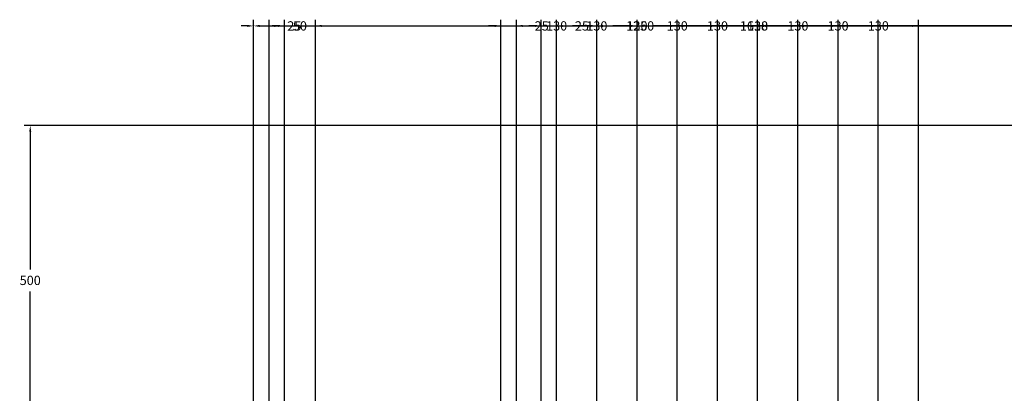
# Model space of a CAD drawing. Units: millimetres. Extents: x 937 to 4561, y 2711 to 5748.
# Tile 4 of 8: x 951 to 2543, y 5145 to 5748. Entities that reach past the tile are written whole.
import ezdxf

# ---------------------------------------------------------------- set-up
doc = ezdxf.new("R2010")
doc.units = ezdxf.units.MM
doc.header["$MEASUREMENT"] = 0
doc.layers.add('A-ANNO-DIMS', color=2, linetype='Continuous', lineweight=18)
doc.styles.get("Standard").update_dxf_attribs({"font": 'arial.ttf'})
doc.dimstyles.get("Standard").update_dxf_attribs({"dimtxt": 15, "dimasz": 10, "dimexe": 10, "dimexo": 10, "dimgap": 10, "dimtad": 0, "dimtih": 1, "dimtoh": 1, "dimdec": 0, "dimzin": 0, "dimdsep": 46, "dimtxsty": 'Standard', "dimcen": 5, "dimadec": 0, "dimazin": 0, "dimtfac": 1, "dimtdec": 0, "dimtofl": 0, "dimtmove": 0, "dimatfit": 3, "dimfxl": 1, "dimtolj": 1, "dimtzin": 0, "dimarcsym": 0})

# ---------------------------------------------------------------- blocks, each defined once
blk = doc.blocks.new('*D15')
at = {"layer": 'A-ANNO-DIMS', "color": 0, "lineweight": -2, "transparency": 16777216}
for p, q in [((1329.5, 4086.9), (1329.5, 5747.9)), ((4179.5, 5586.9), (4179.5, 5747.9)), ((1339.5, 5737.9), (2722, 5737.9)), ((4169.5, 5737.9), (2787, 5737.9))]:
    blk.add_line(p, q, dxfattribs=at)
at = {"layer": 'A-ANNO-DIMS', "color": 0, "transparency": 16777216}
for points in [[(1339.5, 5739.6), (1339.5, 5736.2), (1329.5, 5737.9)], [(4169.5, 5739.6), (4169.5, 5736.2), (4179.5, 5737.9)]]:
    blk.add_solid(points, dxfattribs=at)
at = {"layer": 'Defpoints', "color": 0, "transparency": 16777216}
for p in [(4179.5, 5737.9), (4179.5, 5576.9), (1329.5, 4076.9)]:
    blk.add_point(p, dxfattribs=at)
at = {"layer": 'A-ANNO-DIMS', "color": 0, "transparency": 16777216, "insert": (2754.5, 5737.9), "char_height": 15, "attachment_point": 5}
blk.add_mtext('\\A1;2850', dxfattribs=at)
blk = doc.blocks.new('*D16')
at = {"layer": 'A-ANNO-DIMS', "color": 0, "lineweight": -2, "transparency": 16777216}
for p, q in [((1329.5, 4859.2), (1329.5, 5747.9)), ((2947.4, 5137.7), (2947.4, 5747.9)), ((1339.5, 5737.9), (2106.8, 5737.9)), ((2937.4, 5737.9), (2170.2, 5737.9))]:
    blk.add_line(p, q, dxfattribs=at)
at = {"layer": 'A-ANNO-DIMS', "color": 0, "transparency": 16777216}
for points in [[(1339.5, 5739.6), (1339.5, 5736.2), (1329.5, 5737.9)], [(2937.4, 5739.6), (2937.4, 5736.2), (2947.4, 5737.9)]]:
    blk.add_solid(points, dxfattribs=at)
at = {"layer": 'Defpoints', "color": 0, "transparency": 16777216}
for p in [(2947.4, 5737.9), (2947.4, 5127.7), (1329.5, 4849.2)]:
    blk.add_point(p, dxfattribs=at)
at = {"layer": 'A-ANNO-DIMS', "color": 0, "transparency": 16777216, "insert": (2138.5, 5737.9), "char_height": 15, "attachment_point": 5}
blk.add_mtext('\\A1;1618', dxfattribs=at)
blk = doc.blocks.new('*D20')
at = {"layer": 'A-ANNO-DIMS', "color": 0, "lineweight": -2, "transparency": 16777216}
for p, q in [((1379.5, 5086.9), (1379.5, 5747.9)), ((1429.5, 5036.9), (1429.5, 5747.9)), ((1369.5, 5737.9), (1359.5, 5737.9)), ((1439.5, 5737.9), (1449.5, 5737.9))]:
    blk.add_line(p, q, dxfattribs=at)
at = {"layer": 'A-ANNO-DIMS', "color": 0, "transparency": 16777216}
for points in [[(1369.5, 5739.6), (1369.5, 5736.2), (1379.5, 5737.9)], [(1439.5, 5739.6), (1439.5, 5736.2), (1429.5, 5737.9)]]:
    blk.add_solid(points, dxfattribs=at)
at = {"layer": 'Defpoints', "color": 0, "transparency": 16777216}
for p in [(1429.5, 5737.9), (1379.5, 5076.9), (1429.5, 5026.9)]:
    blk.add_point(p, dxfattribs=at)
at = {"layer": 'A-ANNO-DIMS', "color": 0, "transparency": 16777216, "insert": (1404.5, 5737.9), "char_height": 15, "attachment_point": 5}
blk.add_mtext('\\A1;50', dxfattribs=at)
blk = doc.blocks.new('*D21')
at = {"layer": 'A-ANNO-DIMS', "color": 0, "lineweight": -2, "transparency": 16777216}
for p, q in [((1329.5, 4808.5), (1329.5, 5747.9)), ((1354.5, 4787.4), (1354.5, 5747.9)), ((1319.5, 5737.9), (1309.5, 5737.9)), ((1364.5, 5737.9), (1374.5, 5737.9))]:
    blk.add_line(p, q, dxfattribs=at)
at = {"layer": 'A-ANNO-DIMS', "color": 0, "transparency": 16777216}
for points in [[(1319.5, 5739.6), (1319.5, 5736.2), (1329.5, 5737.9)], [(1364.5, 5739.6), (1364.5, 5736.2), (1354.5, 5737.9)]]:
    blk.add_solid(points, dxfattribs=at)
at = {"layer": 'Defpoints', "color": 0, "transparency": 16777216}
for p in [(1354.5, 5737.9), (1329.5, 4798.5), (1354.5, 4777.4)]:
    blk.add_point(p, dxfattribs=at)
at = {"layer": 'A-ANNO-DIMS', "color": 0, "transparency": 16777216, "insert": (1395.4, 5737.9), "char_height": 15, "attachment_point": 5}
blk.add_mtext('\\A1;25', dxfattribs=at)
blk = doc.blocks.new('*D30')
at = {"layer": 'A-ANNO-DIMS', "color": 0, "lineweight": -2, "transparency": 16777216}
for p, q in [((1794.5, 4411.9), (1794.5, 5747.9)), ((1819.5, 4436.9), (1819.5, 5747.9)), ((1784.5, 5737.9), (1774.5, 5737.9)), ((1829.5, 5737.9), (1839.5, 5737.9))]:
    blk.add_line(p, q, dxfattribs=at)
at = {"layer": 'A-ANNO-DIMS', "color": 0, "transparency": 16777216}
for points in [[(1784.5, 5739.6), (1784.5, 5736.2), (1794.5, 5737.9)], [(1829.5, 5739.6), (1829.5, 5736.2), (1819.5, 5737.9)]]:
    blk.add_solid(points, dxfattribs=at)
at = {"layer": 'Defpoints', "color": 0, "transparency": 16777216}
for p in [(1819.5, 5737.9), (1819.5, 4426.9), (1794.5, 4401.9)]:
    blk.add_point(p, dxfattribs=at)
at = {"layer": 'A-ANNO-DIMS', "color": 0, "transparency": 16777216, "insert": (1860.4, 5737.9), "char_height": 15, "attachment_point": 5}
blk.add_mtext('\\A1;25', dxfattribs=at)
blk = doc.blocks.new('*D31')
at = {"layer": 'A-ANNO-DIMS', "color": 0, "lineweight": -2, "transparency": 16777216}
for p, q in [((1819.5, 4436.9), (1819.5, 5747.9)), ((1949.5, 4436.9), (1949.5, 5747.9)), ((1829.5, 5737.9), (1858.6, 5737.9)), ((1939.5, 5737.9), (1910.3, 5737.9))]:
    blk.add_line(p, q, dxfattribs=at)
at = {"layer": 'A-ANNO-DIMS', "color": 0, "transparency": 16777216}
for points in [[(1829.5, 5739.6), (1829.5, 5736.2), (1819.5, 5737.9)], [(1939.5, 5739.6), (1939.5, 5736.2), (1949.5, 5737.9)]]:
    blk.add_solid(points, dxfattribs=at)
at = {"layer": 'Defpoints', "color": 0, "transparency": 16777216}
for p in [(1949.5, 5737.9), (1819.5, 4426.9), (1949.5, 4426.9)]:
    blk.add_point(p, dxfattribs=at)
at = {"layer": 'A-ANNO-DIMS', "color": 0, "transparency": 16777216, "insert": (1884.5, 5737.9), "char_height": 15, "attachment_point": 5}
blk.add_mtext('\\A1;130', dxfattribs=at)
blk = doc.blocks.new('*D32')
at = {"layer": 'A-ANNO-DIMS', "color": 0, "lineweight": -2, "transparency": 16777216}
for p, q in [((1949.5, 4436.9), (1949.5, 5747.9)), ((2079.5, 4436.9), (2079.5, 5747.9)), ((1959.5, 5737.9), (1988.6, 5737.9)), ((2069.5, 5737.9), (2040.3, 5737.9))]:
    blk.add_line(p, q, dxfattribs=at)
at = {"layer": 'A-ANNO-DIMS', "color": 0, "transparency": 16777216}
for points in [[(1959.5, 5739.6), (1959.5, 5736.2), (1949.5, 5737.9)], [(2069.5, 5739.6), (2069.5, 5736.2), (2079.5, 5737.9)]]:
    blk.add_solid(points, dxfattribs=at)
at = {"layer": 'Defpoints', "color": 0, "transparency": 16777216}
for p in [(2079.5, 5737.9), (1949.5, 4426.9), (2079.5, 4426.9)]:
    blk.add_point(p, dxfattribs=at)
at = {"layer": 'A-ANNO-DIMS', "color": 0, "transparency": 16777216, "insert": (2014.5, 5737.9), "char_height": 15, "attachment_point": 5}
blk.add_mtext('\\A1;130', dxfattribs=at)
blk = doc.blocks.new('*D33')
at = {"layer": 'A-ANNO-DIMS', "color": 0, "lineweight": -2, "transparency": 16777216}
for p, q in [((2079.5, 4436.9), (2079.5, 5747.9)), ((2209.5, 4436.9), (2209.5, 5747.9)), ((2089.5, 5737.9), (2118.6, 5737.9)), ((2199.5, 5737.9), (2170.3, 5737.9))]:
    blk.add_line(p, q, dxfattribs=at)
at = {"layer": 'A-ANNO-DIMS', "color": 0, "transparency": 16777216}
for points in [[(2089.5, 5739.6), (2089.5, 5736.2), (2079.5, 5737.9)], [(2199.5, 5739.6), (2199.5, 5736.2), (2209.5, 5737.9)]]:
    blk.add_solid(points, dxfattribs=at)
at = {"layer": 'Defpoints', "color": 0, "transparency": 16777216}
for p in [(2209.5, 5737.9), (2079.5, 4426.9), (2209.5, 4426.9)]:
    blk.add_point(p, dxfattribs=at)
at = {"layer": 'A-ANNO-DIMS', "color": 0, "transparency": 16777216, "insert": (2144.5, 5737.9), "char_height": 15, "attachment_point": 5}
blk.add_mtext('\\A1;130', dxfattribs=at)
blk = doc.blocks.new('*D34')
at = {"layer": 'A-ANNO-DIMS', "color": 0, "lineweight": -2, "transparency": 16777216}
for p, q in [((2209.5, 4436.9), (2209.5, 5747.9)), ((2339.5, 4436.9), (2339.5, 5747.9)), ((2219.5, 5737.9), (2248.6, 5737.9)), ((2329.5, 5737.9), (2300.3, 5737.9))]:
    blk.add_line(p, q, dxfattribs=at)
at = {"layer": 'A-ANNO-DIMS', "color": 0, "transparency": 16777216}
for points in [[(2219.5, 5739.6), (2219.5, 5736.2), (2209.5, 5737.9)], [(2329.5, 5739.6), (2329.5, 5736.2), (2339.5, 5737.9)]]:
    blk.add_solid(points, dxfattribs=at)
at = {"layer": 'Defpoints', "color": 0, "transparency": 16777216}
for p in [(2339.5, 5737.9), (2209.5, 4426.9), (2339.5, 4426.9)]:
    blk.add_point(p, dxfattribs=at)
at = {"layer": 'A-ANNO-DIMS', "color": 0, "transparency": 16777216, "insert": (2274.5, 5737.9), "char_height": 15, "attachment_point": 5}
blk.add_mtext('\\A1;130', dxfattribs=at)
blk = doc.blocks.new('*D37')
at = {"layer": 'A-ANNO-DIMS', "color": 0, "lineweight": -2, "transparency": 16777216}
for p, q in [((1729.5, 3411.9), (1729.5, 5747.9)), ((1754.5, 3436.9), (1754.5, 5747.9)), ((1719.5, 5737.9), (1709.5, 5737.9)), ((1764.5, 5737.9), (1774.5, 5737.9))]:
    blk.add_line(p, q, dxfattribs=at)
at = {"layer": 'A-ANNO-DIMS', "color": 0, "transparency": 16777216}
for points in [[(1719.5, 5739.6), (1719.5, 5736.2), (1729.5, 5737.9)], [(1764.5, 5739.6), (1764.5, 5736.2), (1754.5, 5737.9)]]:
    blk.add_solid(points, dxfattribs=at)
at = {"layer": 'Defpoints', "color": 0, "transparency": 16777216}
for p in [(1754.5, 5737.9), (1754.5, 3426.9), (1729.5, 3401.9)]:
    blk.add_point(p, dxfattribs=at)
at = {"layer": 'A-ANNO-DIMS', "color": 0, "transparency": 16777216, "insert": (1795.4, 5737.9), "char_height": 15, "attachment_point": 5}
blk.add_mtext('\\A1;25', dxfattribs=at)
blk = doc.blocks.new('*D38')
at = {"layer": 'A-ANNO-DIMS', "color": 0, "lineweight": -2, "transparency": 16777216}
for p, q in [((1754.5, 3436.9), (1754.5, 5747.9)), ((1884.5, 3436.9), (1884.5, 5747.9)), ((1764.5, 5737.9), (1793.6, 5737.9)), ((1874.5, 5737.9), (1845.3, 5737.9))]:
    blk.add_line(p, q, dxfattribs=at)
at = {"layer": 'A-ANNO-DIMS', "color": 0, "transparency": 16777216}
for points in [[(1764.5, 5739.6), (1764.5, 5736.2), (1754.5, 5737.9)], [(1874.5, 5739.6), (1874.5, 5736.2), (1884.5, 5737.9)]]:
    blk.add_solid(points, dxfattribs=at)
at = {"layer": 'Defpoints', "color": 0, "transparency": 16777216}
for p in [(1884.5, 5737.9), (1754.5, 3426.9), (1884.5, 3426.9)]:
    blk.add_point(p, dxfattribs=at)
at = {"layer": 'A-ANNO-DIMS', "color": 0, "transparency": 16777216, "insert": (1819.5, 5737.9), "char_height": 15, "attachment_point": 5}
blk.add_mtext('\\A1;130', dxfattribs=at)
blk = doc.blocks.new('*D39')
at = {"layer": 'A-ANNO-DIMS', "color": 0, "lineweight": -2, "transparency": 16777216}
for p, q in [((1884.5, 3436.9), (1884.5, 5747.9)), ((2014.5, 3436.9), (2014.5, 5747.9)), ((1894.5, 5737.9), (1923.6, 5737.9)), ((2004.5, 5737.9), (1975.3, 5737.9))]:
    blk.add_line(p, q, dxfattribs=at)
at = {"layer": 'A-ANNO-DIMS', "color": 0, "transparency": 16777216}
for points in [[(1894.5, 5739.6), (1894.5, 5736.2), (1884.5, 5737.9)], [(2004.5, 5739.6), (2004.5, 5736.2), (2014.5, 5737.9)]]:
    blk.add_solid(points, dxfattribs=at)
at = {"layer": 'Defpoints', "color": 0, "transparency": 16777216}
for p in [(2014.5, 5737.9), (1884.5, 3426.9), (2014.5, 3426.9)]:
    blk.add_point(p, dxfattribs=at)
at = {"layer": 'A-ANNO-DIMS', "color": 0, "transparency": 16777216, "insert": (1949.5, 5737.9), "char_height": 15, "attachment_point": 5}
blk.add_mtext('\\A1;130', dxfattribs=at)
blk = doc.blocks.new('*D40')
at = {"layer": 'A-ANNO-DIMS', "color": 0, "lineweight": -2, "transparency": 16777216}
for p, q in [((2014.5, 3436.9), (2014.5, 5747.9)), ((2144.5, 3436.9), (2144.5, 5747.9)), ((2024.5, 5737.9), (2053.6, 5737.9)), ((2134.5, 5737.9), (2105.3, 5737.9))]:
    blk.add_line(p, q, dxfattribs=at)
at = {"layer": 'A-ANNO-DIMS', "color": 0, "transparency": 16777216}
for points in [[(2024.5, 5739.6), (2024.5, 5736.2), (2014.5, 5737.9)], [(2134.5, 5739.6), (2134.5, 5736.2), (2144.5, 5737.9)]]:
    blk.add_solid(points, dxfattribs=at)
at = {"layer": 'Defpoints', "color": 0, "transparency": 16777216}
for p in [(2144.5, 5737.9), (2014.5, 3426.9), (2144.5, 3426.9)]:
    blk.add_point(p, dxfattribs=at)
at = {"layer": 'A-ANNO-DIMS', "color": 0, "transparency": 16777216, "insert": (2079.5, 5737.9), "char_height": 15, "attachment_point": 5}
blk.add_mtext('\\A1;130', dxfattribs=at)
blk = doc.blocks.new('*D41')
at = {"layer": 'A-ANNO-DIMS', "color": 0, "lineweight": -2, "transparency": 16777216}
for p, q in [((2144.5, 3436.9), (2144.5, 5747.9)), ((2274.5, 3436.9), (2274.5, 5747.9)), ((2154.5, 5737.9), (2183.6, 5737.9)), ((2264.5, 5737.9), (2235.3, 5737.9))]:
    blk.add_line(p, q, dxfattribs=at)
at = {"layer": 'A-ANNO-DIMS', "color": 0, "transparency": 16777216}
for points in [[(2154.5, 5739.6), (2154.5, 5736.2), (2144.5, 5737.9)], [(2264.5, 5739.6), (2264.5, 5736.2), (2274.5, 5737.9)]]:
    blk.add_solid(points, dxfattribs=at)
at = {"layer": 'Defpoints', "color": 0, "transparency": 16777216}
for p in [(2274.5, 5737.9), (2144.5, 3426.9), (2274.5, 3426.9)]:
    blk.add_point(p, dxfattribs=at)
at = {"layer": 'A-ANNO-DIMS', "color": 0, "transparency": 16777216, "insert": (2209.5, 5737.9), "char_height": 15, "attachment_point": 5}
blk.add_mtext('\\A1;130', dxfattribs=at)
blk = doc.blocks.new('*D42')
at = {"layer": 'A-ANNO-DIMS', "color": 0, "lineweight": -2, "transparency": 16777216}
for p, q in [((2274.5, 3436.9), (2274.5, 5747.9)), ((2404.5, 3436.9), (2404.5, 5747.9)), ((2284.5, 5737.9), (2313.6, 5737.9)), ((2394.5, 5737.9), (2365.3, 5737.9))]:
    blk.add_line(p, q, dxfattribs=at)
at = {"layer": 'A-ANNO-DIMS', "color": 0, "transparency": 16777216}
for points in [[(2284.5, 5739.6), (2284.5, 5736.2), (2274.5, 5737.9)], [(2394.5, 5739.6), (2394.5, 5736.2), (2404.5, 5737.9)]]:
    blk.add_solid(points, dxfattribs=at)
at = {"layer": 'Defpoints', "color": 0, "transparency": 16777216}
for p in [(2404.5, 5737.9), (2274.5, 3426.9), (2404.5, 3426.9)]:
    blk.add_point(p, dxfattribs=at)
at = {"layer": 'A-ANNO-DIMS', "color": 0, "transparency": 16777216, "insert": (2339.5, 5737.9), "char_height": 15, "attachment_point": 5}
blk.add_mtext('\\A1;130', dxfattribs=at)
blk = doc.blocks.new('*D43')
at = {"layer": 'A-ANNO-DIMS', "color": 0, "lineweight": -2, "transparency": 16777216}
for p, q in [((1329.5, 4086.9), (1329.5, 5747.9)), ((2579.5, 4086.9), (2579.5, 5747.9)), ((1339.5, 5737.9), (1922.8, 5737.9)), ((2569.5, 5737.9), (1986.2, 5737.9))]:
    blk.add_line(p, q, dxfattribs=at)
at = {"layer": 'A-ANNO-DIMS', "color": 0, "transparency": 16777216}
for points in [[(1339.5, 5739.6), (1339.5, 5736.2), (1329.5, 5737.9)], [(2569.5, 5739.6), (2569.5, 5736.2), (2579.5, 5737.9)]]:
    blk.add_solid(points, dxfattribs=at)
at = {"layer": 'Defpoints', "color": 0, "transparency": 16777216}
for p in [(2579.5, 5737.9), (1329.5, 4076.9), (2579.5, 4076.9)]:
    blk.add_point(p, dxfattribs=at)
at = {"layer": 'A-ANNO-DIMS', "color": 0, "transparency": 16777216, "insert": (1954.5, 5737.9), "char_height": 15, "attachment_point": 5}
blk.add_mtext('\\A1;1250', dxfattribs=at)
blk = doc.blocks.new('*D63')
at = {"layer": 'A-ANNO-DIMS', "color": 0, "lineweight": -2, "transparency": 16777216}
for p, q in [((3169.5, 5576.9), (958.5, 5576.9)), ((968.5, 5566.9), (968.5, 5344.6)), ((968.5, 5086.9), (968.5, 5309.2)), ((1419.5, 5076.9), (958.5, 5076.9))]:
    blk.add_line(p, q, dxfattribs=at)
at = {"layer": 'A-ANNO-DIMS', "color": 0, "transparency": 16777216}
for points in [[(966.8, 5566.9), (970.2, 5566.9), (968.5, 5576.9)], [(966.8, 5086.9), (970.2, 5086.9), (968.5, 5076.9)]]:
    blk.add_solid(points, dxfattribs=at)
at = {"layer": 'Defpoints', "color": 0, "transparency": 16777216}
for p in [(968.5, 5576.9), (3179.5, 5576.9), (1429.5, 5076.9)]:
    blk.add_point(p, dxfattribs=at)
at = {"layer": 'A-ANNO-DIMS', "color": 0, "transparency": 16777216, "insert": (968.5, 5326.9), "char_height": 15, "attachment_point": 5}
blk.add_mtext('\\A1;500', dxfattribs=at)

msp = doc.modelspace()

# ---------------------------------------------------------------- dimensions: what is measured, and where the dimension line sits
at = {"layer": 'A-ANNO-DIMS'}
for base, p1, p2, picture, middle in [((1354.4852, 5737.9013), (1329.4852, 4798.5021), (1354.4852, 4777.437), '*D21', (1395.4129, 5737.9013)), ((4179.4852, 5737.9013), (1329.4852, 4076.9013), (4179.4852, 5576.9013), '*D15', (2754.4852, 5737.9013)), ((2947.4456, 5737.9013), (1329.4852, 4849.2371), (2947.4456, 5127.6834), '*D16', (2138.4654, 5737.9013)), ((2579.4852, 5737.9013), (1329.4852, 4076.9013), (2579.4852, 4076.9013), '*D43', (1954.4852, 5737.9013)), ((1429.4852, 5737.9013), (1379.4852, 5076.9013), (1429.4852, 5026.9013), '*D20', (1404.4852, 5737.9013)), ((1754.4852, 5737.9013), (1729.4852, 3401.9013), (1754.4852, 3426.9013), '*D37', (1795.4129, 5737.9013)), ((1884.4852, 5737.9013), (1754.4852, 3426.9013), (1884.4852, 3426.9013), '*D38', (1819.4852, 5737.9013)), ((1819.4852, 5737.9013), (1794.4852, 4401.9013), (1819.4852, 4426.9013), '*D30', (1860.4129, 5737.9013)), ((1949.4852, 5737.9013), (1819.4852, 4426.9013), (1949.4852, 4426.9013), '*D31', (1884.4852, 5737.9013)), ((2014.4852, 5737.9013), (1884.4852, 3426.9013), (2014.4852, 3426.9013), '*D39', (1949.4852, 5737.9013)), ((2079.4852, 5737.9013), (1949.4852, 4426.9013), (2079.4852, 4426.9013), '*D32', (2014.4852, 5737.9013)), ((2144.4852, 5737.9013), (2014.4852, 3426.9013), (2144.4852, 3426.9013), '*D40', (2079.4852, 5737.9013)), ((2209.4852, 5737.9013), (2079.4852, 4426.9013), (2209.4852, 4426.9013), '*D33', (2144.4852, 5737.9013)), ((2274.4852, 5737.9013), (2144.4852, 3426.9013), (2274.4852, 3426.9013), '*D41', (2209.4852, 5737.9013)), ((2339.4852, 5737.9013), (2209.4852, 4426.9013), (2339.4852, 4426.9013), '*D34', (2274.4852, 5737.9013)), ((2404.4852, 5737.9013), (2274.4852, 3426.9013), (2404.4852, 3426.9013), '*D42', (2339.4852, 5737.9013))]:
    dim = msp.add_linear_dim(base=base, p1=p1, p2=p2, dimstyle='Standard', override={"dimdec": 0, "dimlfac": 1, "dimrnd": 0, "dimzin": 0, "dimdsep": 46, "dimlunit": 2}, dxfattribs=at)
    dim.commit()
    dim.dimension.update_dxf_attribs({"geometry": picture, "text_midpoint": middle})
dim = msp.add_linear_dim(base=(968.4852, 5576.9013), p1=(1429.4852, 5076.9013), p2=(3179.4852, 5576.9013), angle=90, dimstyle='Standard', override={"dimdec": 0, "dimlfac": 1, "dimrnd": 0, "dimzin": 0, "dimdsep": 46, "dimlunit": 2}, dxfattribs=at)
dim.commit()
dim.dimension.update_dxf_attribs({"geometry": '*D63', "text_midpoint": (968.4852, 5326.9013)})

doc.saveas('drawing.dxf')
